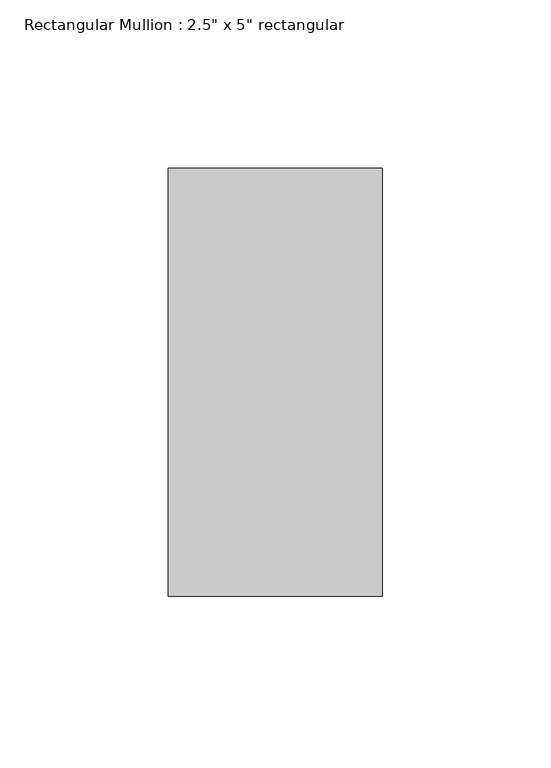
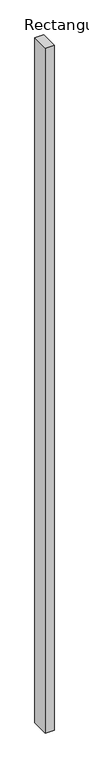
"""IFC4 building model written with IfcOpenShell, lengths in millimetres: member geometry."""

from ifc_helpers import new_model, si_unit, frame, origin, place, context, project, spatial, polyline, outline, extrude, source, transform, mapped, element, save


def member_9c0893e9(model_context):
    return source(origin(), model_context, "Body", "SweptSolid", [
        extrude(outline(polyline([(0.0, 63.5), (0.0, -63.5), (-63.5, -63.5), (-63.5, 63.5), (0.0, 63.5)])), frame((0.0, 0.0, -5183.143409), z_axis=(0.0, 0.0, 1.0), x_axis=(1.0, 0.0, 0.0)), (0.0, 0.0, 1.0), 5183.143409),
    ])


if __name__ == "__main__":
    model = new_model("IFC4")
    model_context = context("Model", 3, world=origin())
    ifc_project = project(units=[si_unit("LENGTHUNIT", "METRE", prefix="MILLI")], contexts=[model_context])
    site = spatial("IfcSite", under=ifc_project)
    building = spatial("IfcBuilding", under=site)
    placement = place(None, origin())
    member_shape = member_9c0893e9(model_context)
    element("IfcMember", 1, ObjectType="Rectangular Mullion : 2.5\" x 5\" rectangular", at=placement, inside=building, context=model_context, shape_type="MappedRepresentation", body=[
        mapped(member_shape, transform((0.0, 0.0, 0.0), x_axis=(1.0, 0.0, 0.0), y_axis=(0.0, 1.0, 0.0), z_axis=(0.0, 0.0, 1.0))),
    ])
    save(model, "model.ifc")

# Revit data of these elements
# Type "Rectangular Mullion : 2.5\" x 5\" rectangular"
#   built-in parameter 1007304 = 0.416667 (stored number, unit not read)
#   built-in parameter 1007301 = 0.104167 (stored number, unit not read)
#   built-in parameter 1007300 = 0.104167 (stored number, unit not read)
# Element 1 (IfcMember, "Rectangular Mullion : 2.5\" x 5\" rectangular")
#   Materials on its faces: "Aluminum"
# Materials
#   "Aluminum": class "Metal", colour RGB 247 247 247, transparency 0, Description = "Aluminum 6061", Cost = 0
